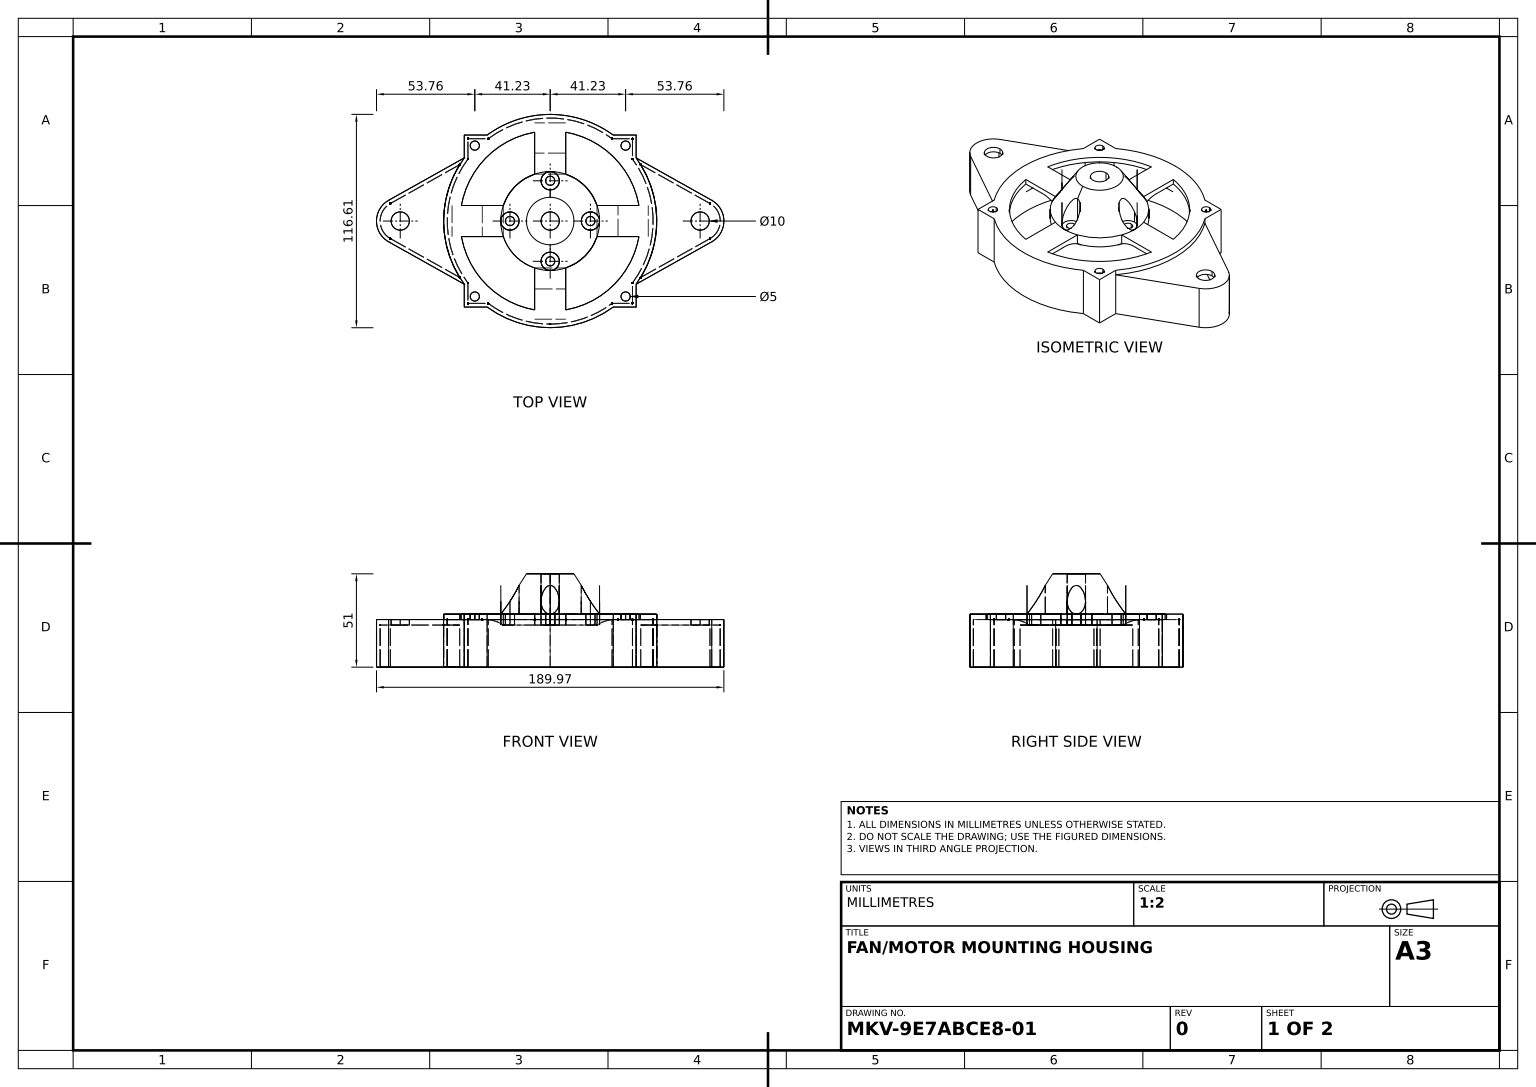
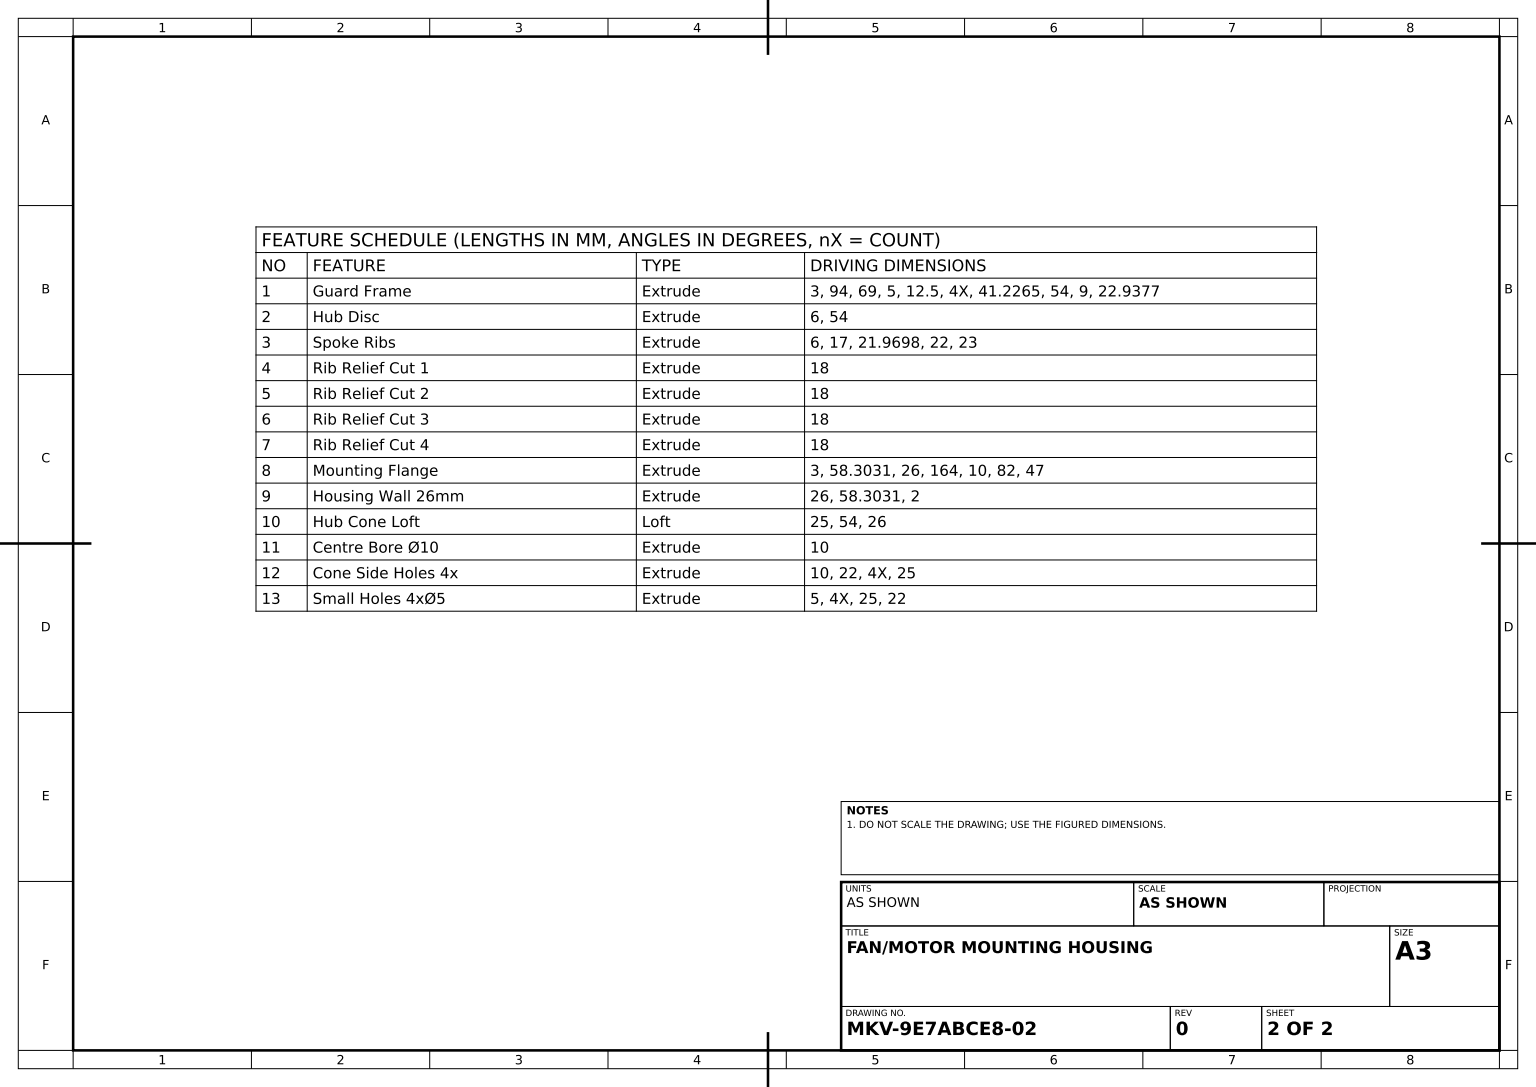
SolidWorks part; units mm, degrees
material "Plain Carbon Steel"
ref_plane "Front Plane" through (0, 0, 0) normal (0, 0, 1) x (1, 0, 0)
ref_plane "Top Plane" through (0, 0, 0) normal (0, 1, 0) x (1, 0, 0)
ref_plane "Right Plane" through (0, 0, 0) normal (1, 0, 0) x (0, 0, -1)
sketch "Guard Frame Sketch" plane through (0, 0, 0) normal (0, 1, 0) x (1, 0, 0)
  line L1 (-47, -47) -> (-34.5, -47)
  line L2 (-47, -47) -> (-47, -34.5)
  line L3 (-47, 47) -> (-34.5, 47)
  line L4 (47, -47) -> (47, -34.5)
  line L5 (-47, -47) -> (47, 47) construction
  line L6 (-47, 47) -> (47, -47) construction
  line L9 (34.5, 47) -> (47, 47)
  line L10 (-47, 34.5) -> (-47, 47)
  line L11 (47, 34.5) -> (47, 47)
  line L12 (34.5, -47) -> (47, -47)
  line L13 (-8.5, 25.6271) -> (-8.5, 48.5648)
  line L14 (8.5, 25.6271) -> (8.5, 48.5648)
  line L15 (25.6271, 8.5) -> (48.5648, 8.5)
  line L16 (25.6271, -8.5) -> (48.5648, -8.5)
  line L17 (8.5, -25.6271) -> (8.5, -48.5648)
  line L18 (-8.5, -25.6271) -> (-8.5, -48.5648)
  line L19 (-25.6271, -8.5) -> (-48.5648, -8.5)
  line L20 (-25.6271, 8.5) -> (-48.5648, 8.5)
  arc A1 (-47, 34.5) -> (-47, -34.5) centre (0, 0) ccw
  circle A2 centre (-41.2265, 41.2265) radius 2.5
  arc A3 (-34.5, -47) -> (34.5, -47) centre (0, 0) ccw
  arc A4 (47, -34.5) -> (47, 34.5) centre (0, 0) ccw
  arc A5 (34.5, 47) -> (-34.5, 47) centre (0, 0) ccw
  circle A6 centre (41.2265, 41.2265) radius 2.5
  circle A7 centre (41.2265, -41.2265) radius 2.5
  circle A8 centre (-41.2265, -41.2265) radius 2.5
  arc A10 (-8.5, 48.5648) -> (-48.5648, 8.5) centre (0, 0) ccw
  circle A11 centre (0, 0) radius 27
  arc A12 (-48.5648, -8.5) -> (-8.5, -48.5648) centre (0, 0) ccw
  arc A13 (8.5, -48.5648) -> (48.5648, -8.5) centre (0, 0) ccw
  arc A14 (48.5648, 8.5) -> (8.5, 48.5648) centre (0, 0) ccw
  point P0 (0, 0)
  dimension "D1" = 94
  dimension "D2" = 69
  dimension "D4" = 5
  dimension "D8" = 54
  dimension "D9" = 22.9377
  dimension "D10" = 9
  dimension "D3" = 12.5
  dimension "D5" = 4
  dimension "D6" = 41.2265
  dimension "D7" = 41.2265
  dimension "D11" = 4
  dimension "D12" = 22.9377
extrude "Guard Frame" add sketch "Guard Frame Sketch" along normal blind 3 contours L9 A5 L3 L10 A1 L2 L1 A3 L12 L4 A4 L11 A14 L15 A11 L16 A13 L17 L18 A12 L19 L20 A10 L13 L14 A8 A7 A6 A2 | A11
sketch "Hub Disc Sketch" plane through (0, 3, 0) normal (0, 1, 0) x (1, 0, 0)
  circle A0 centre (0, 0) radius 27
  dimension "D1" = 54
extrude "Hub Disc" add sketch "Hub Disc Sketch" against normal blind 6
sketch "Spoke Ribs Sketch" plane through (0, 3, 0) normal (0, 1, 0) x (1, 0, 0)
  line L0 (-25.6271, 8.5) -> (-48.5648, 8.5) construction
  line L1 (-37.096, 8.5) -> (-15.1262, 8.5)
  line L2 (-37.096, 8.5) -> (-37.096, -8.5)
  line L3 (-37.096, -8.5) -> (-15.1262, -8.5)
  line L4 (-15.1262, 8.5) -> (-15.1262, -8.5)
  line L5 (-8.5, 25.6271) -> (-8.5, 48.5648) construction
  line L6 (-8.5, 37.096) -> (8.5, 37.096)
  line L7 (-8.5, 37.096) -> (-8.5, 15.096)
  line L8 (-8.5, 15.096) -> (8.5, 15.096)
  line L9 (8.5, 37.096) -> (8.5, 15.096)
  line L10 (25.6271, 8.5) -> (48.5648, 8.5) construction
  line L11 (37.096, 8.5) -> (14.096, 8.5)
  line L12 (37.096, 8.5) -> (37.096, -8.5)
  line L13 (37.096, -8.5) -> (14.096, -8.5)
  line L14 (14.096, 8.5) -> (14.096, -8.5)
  line L15 (-8.5, -25.6271) -> (-8.5, -48.5648) construction
  line L16 (-8.5, -37.096) -> (8.5, -37.096)
  line L17 (-8.5, -37.096) -> (-8.5, -15.096)
  line L18 (-8.5, -15.096) -> (8.5, -15.096)
  line L19 (8.5, -37.096) -> (8.5, -15.096)
  dimension "D1" = 17
  dimension "D2" = 21.9698
  dimension "D3" = 17
  dimension "D4" = 22
  dimension "D5" = 17
  dimension "D6" = 23
  dimension "D7" = 22
  dimension "D8" = 17
extrude "Spoke Ribs" add sketch "Spoke Ribs Sketch" against normal blind 6
sketch "Rib Relief Cut 1 Sketch" plane through (0, 0, 8.5) normal (0, 0, 1) x (1, 0, 0)
  line L0 (-37.096, 0) -> (-37.096, -3)
  line L1 (-37.096, -3) -> (-25.6271, -3)
  arc A0 (-37.096, 0) -> (-25.6271, -3) centre (-35.6626, -17.9428) cw
  dimension "D1" = 18
extrude "Rib Relief Cut 1" cut sketch "Rib Relief Cut 1 Sketch" against normal up to surface (17 mm away) up to face at (-37.096, 0, -8.5)
sketch "Rib Relief Cut 2 Sketch" plane through (-8.5, 0, 0) normal (-1, 0, 0) x (0, 0, 1)
  line L0 (-37.096, 0) -> (-37.096, -3)
  line L1 (-37.096, -3) -> (-25.6271, -3)
  arc A0 (-37.096, 0) -> (-25.6271, -3) centre (-35.6626, -17.9428) cw
  dimension "D1" = 18
extrude "Rib Relief Cut 2" cut sketch "Rib Relief Cut 2 Sketch" against normal up to surface (17 mm away) up to face at (8.5, 0, -37.096)
sketch "Rib Relief Cut 3 Sketch" plane through (0, 0, -8.5) normal (0, 0, -1) x (-1, 0, 0)
  line L0 (-37.096, 0) -> (-37.096, -3)
  line L1 (-37.096, -3) -> (-25.6271, -3)
  arc A0 (-37.096, 0) -> (-25.6271, -3) centre (-35.6626, -17.9428) cw
  dimension "D1" = 18
extrude "Rib Relief Cut 3" cut sketch "Rib Relief Cut 3 Sketch" against normal up to surface (17 mm away) up to face at (37.096, 0, 8.5)
sketch "Rib Relief Cut 4 Sketch" plane through (8.5, 0, 0) normal (1, 0, 0) x (0, 0, -1)
  line L0 (-37.096, 0) -> (-37.096, -3)
  line L1 (-37.096, -3) -> (-25.6271, -3)
  arc A0 (-37.096, 0) -> (-25.6271, -3) centre (-35.6626, -17.9428) cw
  dimension "D1" = 18
extrude "Rib Relief Cut 4" cut sketch "Rib Relief Cut 4 Sketch" against normal up to surface (17 mm away) up to face at (-8.5, 0, 37.096)
sketch "Mounting Flange Sketch" plane through (0, 0, 0) normal (0, -1, 0) x (1, 0, 0)
  line L8 (-47, 34.5) -> (-88.3519, 11.3425)
  line L9 (-47, -34.5) -> (-88.3519, -11.3425)
  line L10 (47, 34.5) -> (88.3519, 11.3425)
  line L11 (47, -34.5) -> (88.3519, -11.3425)
  line L12 (-47, 47) -> (-34.5, 47) construction
  line L14 (34.5, 47) -> (47, 47) construction
  arc A1 (-47, 34.5) -> (-47, -34.5) centre (0, 0) ccw
  arc A3 (47, -34.5) -> (47, 34.5) centre (0, 0) ccw
  arc A4 (-88.3519, 11.3425) -> (-88.3519, -11.3425) centre (-82, 0) ccw
  arc A5 (88.3519, -11.3425) -> (88.3519, 11.3425) centre (82, 0) ccw
  circle A6 centre (-82, 0) radius 5
  circle A7 centre (82, 0) radius 5
  dimension "D1" = 58.3031
  dimension "D2" = 82
  dimension "D3" = 58.3031
  dimension "D4" = 47
  dimension "D5" = 26
  dimension "D6" = 26
  dimension "D10" = 10
  dimension "D9" = 10
  dimension "D7" = 164
  dimension "D8" = 47
extrude "Mounting Flange" add sketch "Mounting Flange Sketch" along normal blind 3 separate body
sketch "Housing Wall Sketch" plane through (0, 0, 0) normal (0, -1, 0) x (1, 0, 0)
  line L0 (-88.3519, 11.3425) -> (-47, 34.5)
  line L1 (-47, 34.5) -> (-47, 47)
  line L2 (-47, 47) -> (-34.5, 47)
  line L3 (34.5, 47) -> (47, 47)
  line L4 (47, 47) -> (47, 34.5)
  line L5 (34.5, -47) -> (47, -47)
  line L6 (47, -47) -> (47, -34.5)
  line L7 (-47, -34.5) -> (-47, -47)
  line L8 (-47, -47) -> (-34.5, -47)
  line L9 (47, 34.5) -> (88.3519, 11.3425)
  line L10 (88.3519, -11.3425) -> (47, -34.5)
  line L11 (-88.3519, -11.3425) -> (-47, -34.5)
  line L12 (-45, 33.8384) -> (-45, 45)
  line L13 (-45, 45) -> (-33.8384, 45)
  line L14 (33.8384, 45) -> (45, 45)
  line L15 (45, 45) -> (45, 33.8384)
  line L16 (-45, 34.5) -> (-45, 45) construction
  line L17 (45, 45) -> (45, 34.5) construction
  line L18 (-45, -33.8384) -> (-45, -45)
  line L19 (-45, -45) -> (-33.8384, -45)
  line L20 (33.8384, -45) -> (45, -45)
  line L21 (45, -45) -> (45, -33.8384)
  line L22 (-45, -34.5) -> (-45, -45) construction
  line L23 (45, -45) -> (45, -34.5) construction
  line L24 (-87.3747, -9.5975) -> (-49.4982, -30.8087)
  line L25 (-87.3747, 9.5975) -> (-49.4982, 30.8087)
  line L26 (49.4982, 30.8087) -> (87.3747, 9.5975)
  line L27 (87.3747, -9.5975) -> (49.4982, -30.8087)
  line L29 (-87.3747, 9.5975) -> (-46.0228, 32.755) construction
  line L30 (-87.3747, -9.5975) -> (-46.0228, -32.755) construction
  line L31 (46.0228, 32.755) -> (87.3747, 9.5975) construction
  line L32 (87.3747, -9.5975) -> (46.0228, -32.755) construction
  arc A0 (-34.5, 47) -> (34.5, 47) centre (0, 0) cw
  arc A1 (47, 34.5) -> (47, -34.5) centre (0, 0) cw
  arc A2 (-34.5, -47) -> (34.5, -47) centre (0, 0) ccw
  arc A3 (-47, -34.5) -> (-47, 34.5) centre (0, 0) cw
  arc A4 (-88.3519, 11.3425) -> (-88.3519, -11.3425) centre (-82, 0) ccw
  arc A5 (88.3519, 11.3425) -> (88.3519, -11.3425) centre (82, 0) cw
  arc A6 (-33.8384, 45) -> (33.8384, 45) centre (0, 0) cw
  arc A7 (-45, -33.8384) -> (-45, 33.8384) centre (0, 0) cw
  arc A8 (45, 33.8384) -> (45, -33.8384) centre (0, 0) cw
  arc A9 (-45.3877, -33.3165) -> (-45.3877, 33.3165) centre (0, 0) cw construction
  arc A10 (45.3877, 33.3165) -> (45.3877, -33.3165) centre (0, 0) cw construction
  arc A11 (-33.8384, -45) -> (33.8384, -45) centre (0, 0) ccw
  arc A12 (-87.3747, 9.5975) -> (-87.3747, -9.5975) centre (-82, 0) ccw
  arc A13 (87.3747, 9.5975) -> (87.3747, -9.5975) centre (82, 0) cw
  line M24 (34.5, -47) -> (47, -47)
  line M25 (47, -47) -> (47, -34.5)
  arc M26 (47, -34.5) -> (47, 34.5) centre (0, 0) ccw
  line M27 (47, 34.5) -> (47, 47)
  line M28 (47, 47) -> (34.5, 47)
  arc M29 (34.5, 47) -> (-34.5, 47) centre (0, 0) ccw
  line M30 (-34.5, 47) -> (-47, 47)
  line M31 (-47, 47) -> (-47, 34.5)
  arc M32 (-47, 34.5) -> (-47, -34.5) centre (0, 0) ccw
  line M33 (-47, -34.5) -> (-47, -47)
  line M34 (-47, -47) -> (-34.5, -47)
  arc M35 (-34.5, -47) -> (34.5, -47) centre (0, 0) ccw
  dimension "D1" = 58.3031
  dimension "D2" = 58.3031
  dimension "D3" = 58.3031
  dimension "D4" = 58.3031
  dimension "D5" = 2
  dimension "D6" = 2
  dimension "D7" = 2
extrude "Housing Wall 26mm" add sketch "Housing Wall Sketch" along normal blind 26 contours A11 L19 L18 A7 L12 L13 A6 L14 L15 A8 L21 L20 M35 M24 M25 M26 M27 M28 M29 M30 M31 M32 M33 M34 | A12 L25 L0 A4 L11 L24 M32 | L26 A13 L27 L10 A5 L9 M26
sketch "Cone Base Circle" plane through (0, 3, 0) normal (0, 1, 0) x (1, 0, 0)
  circle A0 centre (0, 0) radius 27
  dimension "D1" = 54
ref_plane "Cone Top Plane" through (0, 25, 0) normal (0, 1, 0) x (1, 0, 0)
sketch "Cone Top Circle" plane through (0, 25, 0) normal (0, 1, 0) x (1, 0, 0)
  circle A0 centre (0, 0) radius 13
  dimension "D1" = 26
loft "Hub Cone Loft" add profiles "Cone Base Circle", "Cone Top Circle"
sketch "Centre Bore Sketch" plane through (0, 25, 0) normal (0, 1, 0) x (1, 0, 0)
  circle A0 centre (0, 0) radius 5
  dimension "D1" = 10
extrude "Centre Bore Ø10" cut sketch "Centre Bore Sketch" against normal through all
sketch "Cone Side Holes Sketch" plane through (0, 25, 0) normal (0, 1, 0) x (1, 0, 0)
  line L0 (-47, 34.5) -> (-47, 47) construction
  circle A0 centre (0, 22) radius 5
  circle A1 centre (22, 0) radius 5
  circle A3 centre (0, -22) radius 5
  circle A4 centre (-22, 0) radius 5
  dimension "D1" = 10
  dimension "D2" = 22
  dimension "D4" = 22
  dimension "D5" = 25
  dimension "D3" = 4
extrude "Cone Side Holes 4x" cut sketch "Cone Side Holes Sketch" against normal up to surface (22 mm away) up to face at (-41.2265, 3, 43.7265)
sketch "Small Holes Sketch" plane through (0, 3, 0) normal (0, 1, 0) x (1, 0, 0)
  line L0 (-47, 34.5) -> (-47, 47) construction
  circle A0 centre (0, 22) radius 2.5
  circle A1 centre (22, 0) radius 2.5
  circle A2 centre (0, -22) radius 2.5
  circle A3 centre (-22, 0) radius 2.5
  dimension "D1" = 5
  dimension "D3" = 25
  dimension "D4" = 22
  dimension "D2" = 4
extrude "Small Holes 4xØ5" cut sketch "Small Holes Sketch" against normal through all
